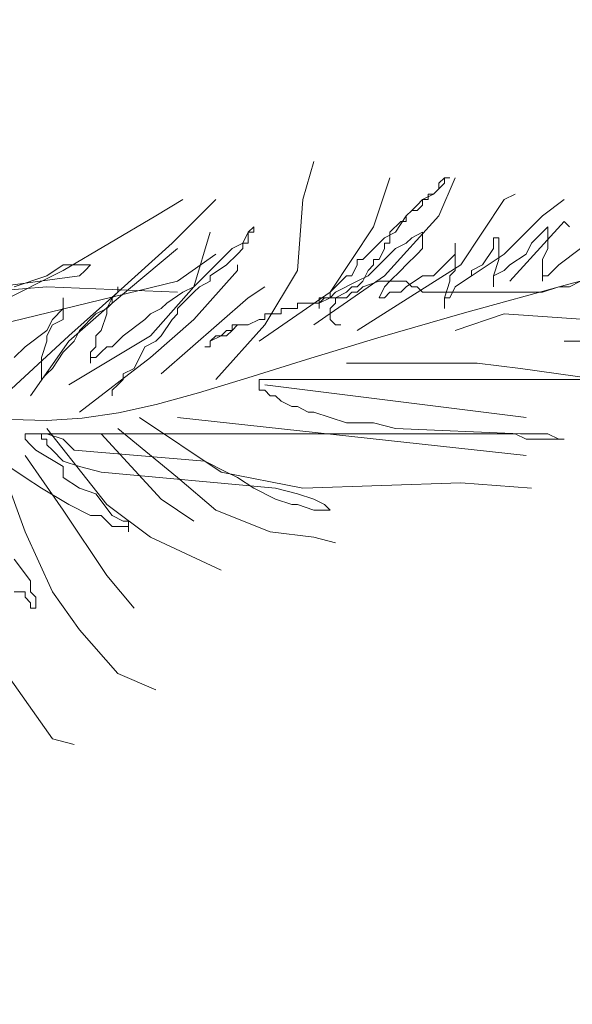
# Model space of a CAD drawing. Units: millimetres. Extents: x 595116 to 630915, y 909473 to 920225.
# Tile 59 of 134: x 629606.022 to 629608.928, y 919290.711 to 919295.882. Entities that reach past the tile are written whole.
import ezdxf

# ---------------------------------------------------------------- set-up
doc = ezdxf.new("R2010")
doc.units = ezdxf.units.MM
doc.layers.add('Dimension', color=3, linetype='Continuous', lineweight=18)
doc.layers.add('L-PLNT', color=85, linetype='Continuous', lineweight=13)
doc.styles.get("Standard").update_dxf_attribs({"font": 'arial.ttf'})
doc.dimstyles.new('ISO-25', dxfattribs={"dimtxt": 9, "dimasz": 6, "dimexe": 1.25, "dimexo": 0.625, "dimtad": 1, "dimlunit": 4, "dimtxsty": 'Standard', "dimcen": 2.5, "dimadec": 0, "dimazin": 0, "dimtfac": 1, "dimtmove": 0, "dimatfit": 3, "dimfxl": 1, "dimarcsym": 0})

# ---------------------------------------------------------------- blocks, each defined once
blk = doc.blocks.new('A$C4FB75ABC')
for p, q in [((4.2249, 2.058), (4.2402, 2.1114)), ((4.324, 2.0199), (4.3469, 2.0885)), ((4.4156, 2.0809), (4.4232, 2.0885)), ((4.4156, 2.0352), (4.4384, 2.0885)), ((4.4156, 2.0733), (4.4156, 2.0809)), ((4.4232, 2.0809), (4.4156, 2.0733)), ((4.4232, 2.0885), (4.4308, 2.0885)), ((4.4308, 2.0885), (4.4232, 2.0885)), ((4.4232, 2.0885), (4.4232, 2.0809)), ((4.4079, 2.0657), (4.4156, 2.0733)), ((4.4156, 2.0733), (4.4079, 2.0657)), ((4.019, 2.0352), (4.0571, 2.058)), ((4.0419, 1.9971), (4.1029, 2.058)), ((4.2173, 1.9589), (4.2249, 2.058)), ((4.3927, 2.058), (4.3851, 2.0504)), ((4.4079, 2.0657), (4.3927, 2.058)), ((4.3927, 2.0504), (4.3927, 2.058)), ((4.3927, 2.058), (4.4003, 2.058)), ((4.4003, 2.058), (4.4003, 2.0657)), ((4.4003, 2.0657), (4.4079, 2.0657)), ((4.4461, 1.9666), (4.5071, 2.058)), ((4.5071, 2.058), (4.5223, 2.0657)), ((4.5605, 2.0352), (4.591, 2.058)), ((4.3698, 2.0352), (4.3774, 2.0428)), ((4.3774, 2.0428), (4.3698, 2.0352)), ((4.3851, 2.0504), (4.3774, 2.0428)), ((4.3774, 2.0428), (4.3851, 2.0428)), ((4.3851, 2.0428), (4.3927, 2.0504)), ((3.8894, 1.9589), (4.019, 2.0352)), ((4.3393, 1.9513), (4.4156, 2.0352)), ((4.3469, 2.0123), (4.3622, 2.0275)), ((4.3698, 2.0352), (4.3546, 2.0123)), ((4.3622, 2.0275), (4.3698, 2.0275)), ((4.3698, 2.0275), (4.3698, 2.0352)), ((4.5071, 1.9818), (4.5605, 2.0352)), ((4.5147, 1.9437), (4.591, 2.0275)), ((4.591, 2.0275), (4.5986, 2.0199)), ((4.0724, 1.9361), (4.0953, 2.0123)), ((4.1486, 2.0123), (4.141, 1.9971)), ((4.1563, 2.0199), (4.1486, 2.0123)), ((4.1486, 1.9971), (4.1486, 2.0123)), ((4.1486, 2.0123), (4.1563, 2.0123)), ((4.1563, 2.0123), (4.1563, 2.0199)), ((4.263, 1.9285), (4.324, 2.0199)), ((4.3546, 2.0123), (4.3393, 2.0047)), ((4.3469, 1.9971), (4.3469, 2.0123)), ((4.3774, 2.0047), (4.3927, 2.0123)), ((4.3927, 2.0123), (4.3927, 1.9894)), ((4.5528, 2.0047), (4.5605, 2.0123)), ((4.5605, 2.0123), (4.5681, 2.0199)), ((4.5681, 2.0199), (4.5681, 1.9894)), ((4.3393, 2.0047), (4.3317, 1.9971)), ((4.3698, 1.9971), (4.3774, 2.0047)), ((4.4918, 1.9894), (4.4918, 2.0047)), ((4.4918, 2.0047), (4.4995, 2.0047)), ((4.4995, 2.0047), (4.4995, 1.9742)), ((4.5452, 1.9971), (4.5528, 2.0047)), ((3.958, 1.9132), (4.0495, 1.9894)), ((3.9656, 1.9285), (4.0419, 1.9971)), ((4.1258, 1.9894), (4.1181, 1.9818)), ((4.141, 1.9971), (4.1258, 1.9894)), ((4.1334, 1.9818), (4.141, 1.9894)), ((4.141, 1.9894), (4.141, 1.9971)), ((4.141, 1.9971), (4.1486, 1.9971)), ((4.3317, 1.9971), (4.3164, 1.9818)), ((4.3317, 1.9742), (4.3393, 1.9894)), ((4.3393, 1.9894), (4.3393, 1.9971)), ((4.3393, 1.9971), (4.3469, 1.9971)), ((4.3469, 1.9818), (4.3546, 1.9894)), ((4.3546, 1.9894), (4.3698, 1.9971)), ((4.3927, 1.9894), (4.3851, 1.9818)), ((4.4384, 1.9818), (4.4384, 1.9971)), ((4.4384, 1.9971), (4.4384, 1.9589)), ((4.4766, 1.9666), (4.4918, 1.9894)), ((4.5376, 1.9818), (4.5452, 1.9971)), ((4.5681, 1.9894), (4.5605, 1.9742)), ((4.5833, 1.9666), (4.6138, 1.9894)), ((4.7725, 1.9851), (4.5975, 1.9398)), ((4.0495, 1.9437), (4.1029, 1.9818)), ((4.1181, 1.9818), (4.1029, 1.9666)), ((4.1181, 1.9666), (4.1334, 1.9818)), ((4.3088, 1.9742), (4.3012, 1.9742)), ((4.3012, 1.9742), (4.3012, 1.9666)), ((4.3164, 1.9818), (4.3088, 1.9742)), ((4.3164, 1.9513), (4.3469, 1.9818)), ((4.324, 1.9666), (4.324, 1.9742)), ((4.324, 1.9742), (4.3317, 1.9742)), ((4.3851, 1.9818), (4.3698, 1.9666)), ((4.4156, 1.9589), (4.4308, 1.9742)), ((4.4308, 1.9742), (4.4384, 1.9818)), ((4.4384, 1.9361), (4.5071, 1.9818)), ((4.4995, 1.9742), (4.4918, 1.9513)), ((4.5147, 1.9666), (4.5376, 1.9818)), ((4.5605, 1.9742), (4.5605, 1.9437)), ((3.7521, 1.8903), (3.8894, 1.9589)), ((3.8894, 1.9666), (3.8665, 1.9513)), ((3.9275, 1.9666), (3.8894, 1.9666)), ((3.9122, 1.9513), (3.9199, 1.9589)), ((3.9199, 1.9589), (3.9275, 1.9666)), ((4.0724, 1.8903), (4.1334, 1.9589)), ((4.1029, 1.9666), (4.08, 1.9437)), ((4.0953, 1.9513), (4.1181, 1.9666)), ((4.1334, 1.9589), (4.1334, 1.9666)), ((4.1715, 1.8827), (4.2173, 1.9589)), ((4.3012, 1.9666), (4.2935, 1.9513)), ((4.3012, 1.8751), (4.4461, 1.9666)), ((4.3088, 1.9437), (4.3164, 1.9589)), ((4.3164, 1.9589), (4.324, 1.9666)), ((4.3622, 1.9589), (4.3469, 1.9437)), ((4.3698, 1.9666), (4.3622, 1.9589)), ((4.4079, 1.9513), (4.4156, 1.9589)), ((4.4384, 1.9589), (4.4308, 1.9513)), ((4.4613, 1.9589), (4.4766, 1.9666)), ((4.4613, 1.9513), (4.4613, 1.9589)), ((4.4918, 1.9513), (4.5071, 1.9589)), ((4.5071, 1.9589), (4.5147, 1.9666)), ((4.5681, 1.9513), (4.5757, 1.9589)), ((4.5757, 1.9589), (4.5833, 1.9666)), ((3.7445, 1.9285), (3.9122, 1.9513)), ((3.7978, 1.8827), (4.0495, 1.9437)), ((3.8665, 1.9513), (3.8207, 1.9361)), ((4.08, 1.9437), (4.0724, 1.9361)), ((4.08, 1.9361), (4.0953, 1.9437)), ((4.0953, 1.9437), (4.0953, 1.9513)), ((4.2402, 1.8827), (4.3393, 1.9513)), ((4.2859, 1.9513), (4.2707, 1.9361)), ((4.2707, 1.9285), (4.3012, 1.9437)), ((4.2935, 1.9513), (4.2859, 1.9513)), ((4.3012, 1.9437), (4.3164, 1.9513)), ((4.3012, 1.9361), (4.3088, 1.9437)), ((4.3317, 1.9437), (4.3088, 1.9361)), ((4.3698, 1.9437), (4.3317, 1.9437)), ((4.3469, 1.9437), (4.3393, 1.9361)), ((4.3698, 1.9361), (4.3927, 1.9513)), ((4.3774, 1.9361), (4.3698, 1.9437)), ((4.3927, 1.9513), (4.4079, 1.9513)), ((4.4308, 1.9437), (4.4232, 1.9208)), ((4.4308, 1.9513), (4.4308, 1.9437)), ((4.4384, 1.9361), (4.4613, 1.9513)), ((4.4918, 1.9513), (4.4918, 1.9361)), ((4.4918, 1.9361), (4.4918, 1.9513)), ((4.5605, 1.9513), (4.5681, 1.9513)), ((4.5605, 1.9437), (4.5605, 1.9513)), ((4.6138, 1.9437), (4.5986, 1.9361)), ((3.5843, 1.9132), (3.8665, 1.9361)), ((3.8665, 1.9361), (4.0495, 1.9285)), ((3.9656, 1.9285), (3.9656, 1.9361)), ((3.9656, 1.9361), (3.9656, 1.9285)), ((4.0114, 1.8675), (4.0724, 1.9361)), ((4.0724, 1.9361), (4.0571, 1.9285)), ((4.0724, 1.9285), (4.08, 1.9361)), ((4.1486, 1.9208), (4.1715, 1.9361)), ((4.2707, 1.9361), (4.263, 1.9285)), ((4.2859, 1.9285), (4.2935, 1.9361)), ((4.2935, 1.9361), (4.3012, 1.9361)), ((4.3088, 1.9361), (4.3012, 1.9285)), ((4.3393, 1.9361), (4.3317, 1.9208)), ((4.3622, 1.9285), (4.3698, 1.9361)), ((4.3851, 1.9361), (4.3774, 1.9361)), ((4.3927, 1.9285), (4.3851, 1.9361)), ((4.4308, 1.9208), (4.4384, 1.9361)), ((4.5975, 1.9398), (4.4513, 1.8996)), ((4.5833, 1.9361), (4.5605, 1.9285)), ((4.5986, 1.9361), (4.5833, 1.9361)), ((3.8894, 1.8903), (3.8894, 1.9208)), ((3.8894, 1.9208), (3.8894, 1.9056)), ((3.897, 1.8675), (3.9656, 1.9285)), ((3.958, 1.9208), (3.9504, 1.9056)), ((3.958, 1.9208), (3.9656, 1.9285)), ((3.9656, 1.9285), (3.958, 1.9208)), ((3.958, 1.9132), (3.958, 1.9208)), ((4.0266, 1.8141), (4.1486, 1.9208)), ((4.0571, 1.9285), (4.0343, 1.9132)), ((4.0571, 1.9132), (4.0724, 1.9285)), ((4.1639, 1.8599), (4.263, 1.9285)), ((4.2554, 1.9208), (4.2478, 1.9132)), ((4.2478, 1.9056), (4.2478, 1.9208)), ((4.2478, 1.9208), (4.263, 1.9208)), ((4.263, 1.9208), (4.2478, 1.9132)), ((4.263, 1.9208), (4.2554, 1.9208)), ((4.263, 1.9285), (4.263, 1.9208)), ((4.263, 1.9208), (4.2707, 1.9285)), ((4.2859, 1.9208), (4.263, 1.9208)), ((4.2707, 1.9208), (4.2859, 1.9285)), ((4.2707, 1.9132), (4.2707, 1.9208)), ((4.2935, 1.9285), (4.2859, 1.9208)), ((4.3012, 1.9285), (4.2935, 1.9285)), ((4.3317, 1.9208), (4.3393, 1.9208)), ((4.3393, 1.9208), (4.3469, 1.9285)), ((4.3469, 1.9285), (4.3622, 1.9285)), ((4.5605, 1.9285), (4.3927, 1.9285)), ((4.4232, 1.9208), (4.4232, 1.9056)), ((4.4232, 1.9056), (4.4232, 1.9208)), ((4.4232, 1.9208), (4.4308, 1.9208)), ((3.8894, 1.9056), (3.8741, 1.8903)), ((3.897, 1.8599), (3.958, 1.9132)), ((3.9504, 1.9056), (3.9351, 1.898)), ((3.9504, 1.9056), (3.958, 1.9132)), ((3.9504, 1.898), (3.9504, 1.9056)), ((4.0266, 1.9056), (4.0114, 1.898)), ((4.0343, 1.9132), (4.0266, 1.9056)), ((4.0495, 1.9056), (4.0571, 1.9132)), ((4.0495, 1.898), (4.0495, 1.9056)), ((4.2173, 1.9056), (4.1944, 1.9056)), ((4.1944, 1.9056), (4.1944, 1.898)), ((4.2478, 1.9132), (4.2173, 1.9132)), ((4.2173, 1.9132), (4.2173, 1.9056)), ((4.2478, 1.9132), (4.2478, 1.9056)), ((4.263, 1.9056), (4.2707, 1.9132)), ((4.263, 1.8903), (4.263, 1.9056)), ((3.8741, 1.8903), (3.8665, 1.8751)), ((3.8741, 1.8827), (3.8894, 1.8903)), ((3.9351, 1.898), (3.9122, 1.8751)), ((3.9427, 1.8751), (3.9504, 1.898)), ((4.0037, 1.8903), (3.9732, 1.8675)), ((4.0114, 1.898), (4.0037, 1.8903)), ((4.0114, 1.837), (4.0724, 1.8903)), ((4.0266, 1.8675), (4.0419, 1.8903)), ((4.0419, 1.8903), (4.0495, 1.898)), ((4.1639, 1.8903), (4.1486, 1.8827)), ((4.1715, 1.8903), (4.1639, 1.8903)), ((4.1944, 1.898), (4.1715, 1.898)), ((4.1715, 1.898), (4.1715, 1.8903)), ((4.2707, 1.8827), (4.263, 1.8903)), ((4.4513, 1.8996), (4.3302, 1.8644)), ((4.4384, 1.8751), (4.5071, 1.898)), ((4.5071, 1.898), (4.6215, 1.8903)), ((3.8665, 1.8751), (3.836, 1.8522)), ((3.8665, 1.8675), (3.8741, 1.8827)), ((3.9122, 1.8751), (3.9046, 1.8599)), ((3.9351, 1.8675), (3.9427, 1.8751)), ((4.1029, 1.8065), (4.1715, 1.8827)), ((4.1181, 1.8751), (4.1105, 1.8675)), ((4.1258, 1.8751), (4.1181, 1.8751)), ((4.1181, 1.8675), (4.1258, 1.8751)), ((4.1334, 1.8827), (4.1258, 1.8751)), ((4.1258, 1.8751), (4.1258, 1.8827)), ((4.1258, 1.8827), (4.1334, 1.8827)), ((4.1486, 1.8827), (4.1334, 1.8827)), ((4.2783, 1.8827), (4.2707, 1.8827)), ((3.7978, 1.776), (3.897, 1.8675)), ((3.8436, 1.7836), (3.897, 1.8599)), ((3.8589, 1.837), (3.8665, 1.8599)), ((3.8665, 1.8599), (3.8665, 1.8675)), ((3.9046, 1.8599), (3.8894, 1.8446)), ((3.897, 1.7989), (4.0114, 1.8675)), ((3.9351, 1.8522), (3.9351, 1.8675)), ((3.9656, 1.8599), (3.958, 1.8522)), ((3.9732, 1.8675), (3.9656, 1.8599)), ((4.0037, 1.8522), (4.019, 1.8599)), ((4.019, 1.8599), (4.0266, 1.8675)), ((4.1029, 1.8675), (4.0953, 1.8599)), ((4.0953, 1.8599), (4.1105, 1.8675)), ((4.0953, 1.8599), (4.0953, 1.8522)), ((4.0953, 1.8522), (4.0953, 1.8599)), ((4.1105, 1.8675), (4.1029, 1.8675)), ((4.1105, 1.8675), (4.1181, 1.8675)), ((4.3302, 1.8644), (4.2303, 1.8341)), ((4.6062, 1.8599), (4.591, 1.8599)), ((4.591, 1.8599), (4.652, 1.8599)), ((3.836, 1.8522), (3.8207, 1.837)), ((3.9275, 1.8446), (3.9351, 1.8522)), ((3.9504, 1.8522), (3.9427, 1.8446)), ((3.958, 1.8522), (3.9504, 1.8522)), ((3.9885, 1.8217), (4.0037, 1.8522)), ((4.0953, 1.8522), (4.0876, 1.8522)), ((4.0876, 1.8522), (4.0953, 1.8522)), ((3.8589, 1.8065), (3.8589, 1.837)), ((3.8894, 1.8446), (3.8741, 1.8217)), ((3.9122, 1.7608), (4.0114, 1.837)), ((3.9275, 1.8294), (3.9275, 1.8446)), ((3.9351, 1.837), (3.9275, 1.837)), ((3.9275, 1.837), (3.9275, 1.8294)), ((3.9427, 1.8446), (3.9351, 1.837)), ((4.2303, 1.8341), (4.1477, 1.8087)), ((3.8741, 1.8217), (3.8665, 1.8141)), ((3.9732, 1.8141), (3.9885, 1.8217)), ((4.2859, 1.8294), (4.4689, 1.8294)), ((4.4689, 1.8294), (4.53, 1.8217)), ((4.53, 1.8217), (4.6367, 1.8065)), ((3.8665, 1.8141), (3.8589, 1.8065)), ((3.9656, 1.7989), (3.9732, 1.8065)), ((3.9732, 1.8065), (3.9732, 1.8141)), ((4.1477, 1.8087), (4.0788, 1.7878)), ((4.1639, 1.7913), (4.1639, 1.8065)), ((4.1639, 1.8065), (5.0333, 1.8065)), ((3.958, 1.7913), (3.9656, 1.7989)), ((3.958, 1.7836), (3.958, 1.7913)), ((4.1715, 1.7913), (4.1639, 1.7913)), ((4.1715, 1.7989), (4.5376, 1.7531)), ((4.1792, 1.7836), (4.1715, 1.7913)), ((4.0788, 1.7878), (4.0197, 1.7715)), ((4.1868, 1.7836), (4.1792, 1.7836)), ((4.1944, 1.776), (4.1868, 1.7836)), ((4.0197, 1.7715), (3.9666, 1.7597)), ((4.2097, 1.7684), (4.1944, 1.776)), ((4.2173, 1.7684), (4.2097, 1.7684)), ((4.2325, 1.7608), (4.2173, 1.7684)), ((3.8664, 1.749), (3.8165, 1.7504)), ((3.916, 1.7521), (3.8664, 1.749)), ((3.9666, 1.7597), (3.916, 1.7521)), ((3.9961, 1.7531), (4.1105, 1.6769)), ((4.0495, 1.7531), (4.5376, 1.6998)), ((4.2402, 1.7608), (4.2325, 1.7608)), ((4.2859, 1.7455), (4.2402, 1.7608)), ((3.8665, 1.7379), (3.9504, 1.6312)), ((3.9656, 1.7379), (4.0495, 1.6693)), ((4.324, 1.7455), (4.2859, 1.7455)), ((4.3546, 1.7379), (4.324, 1.7455)), ((4.53, 1.7303), (4.3546, 1.7379)), ((3.836, 1.7227), (3.836, 1.7303)), ((3.836, 1.7303), (3.8665, 1.7303)), ((3.8436, 1.715), (3.836, 1.7227)), ((3.8589, 1.7227), (3.8589, 1.7303)), ((3.8589, 1.7303), (4.5223, 1.7303)), ((3.8665, 1.7227), (3.8589, 1.7227)), ((3.8665, 1.7303), (3.8894, 1.7227)), ((3.8665, 1.715), (3.8665, 1.7227)), ((3.8894, 1.7227), (3.9046, 1.7074)), ((3.9427, 1.7303), (4.0266, 1.6388)), ((4.5223, 1.7303), (4.5376, 1.7227)), ((4.5681, 1.7303), (4.53, 1.7303)), ((4.5376, 1.7227), (4.591, 1.7227)), ((4.5833, 1.7227), (4.5681, 1.7303)), ((4.591, 1.7227), (4.5833, 1.7227)), ((3.8512, 1.7074), (3.8436, 1.715)), ((3.8741, 1.7074), (3.8665, 1.715)), ((3.836, 1.6998), (3.8894, 1.6236)), ((3.8894, 1.6845), (3.8512, 1.7074)), ((3.8894, 1.6922), (3.8741, 1.7074)), ((3.9046, 1.7074), (4.0876, 1.6922)), ((3.8131, 1.6845), (3.836, 1.6693)), ((3.9122, 1.6845), (3.8894, 1.6922)), ((3.8894, 1.6693), (3.8894, 1.6845)), ((3.9427, 1.6769), (3.9122, 1.6845)), ((4.0876, 1.6922), (4.1181, 1.6769)), ((3.8055, 1.6769), (3.836, 1.5931)), ((3.836, 1.6693), (3.8589, 1.6541)), ((3.9122, 1.6541), (3.8894, 1.6693)), ((4.1868, 1.6541), (3.9427, 1.6769)), ((4.0495, 1.6693), (4.1029, 1.6236)), ((4.1105, 1.6769), (4.2249, 1.6541)), ((4.1181, 1.6769), (4.1334, 1.6693)), ((4.1334, 1.6693), (4.1563, 1.6541)), ((3.8589, 1.6541), (3.897, 1.6312)), ((3.9351, 1.6464), (3.9122, 1.6541)), ((4.1563, 1.6541), (4.1868, 1.6388)), ((4.2173, 1.6464), (4.1868, 1.6541)), ((4.2249, 1.6541), (4.4461, 1.6617)), ((4.4461, 1.6617), (4.5452, 1.6541)), ((3.958, 1.6159), (3.9351, 1.6464)), ((4.2402, 1.6388), (4.2173, 1.6464)), ((3.897, 1.6312), (3.9275, 1.6159)), ((3.9504, 1.6312), (4.0114, 1.5855)), ((4.0266, 1.6388), (4.0724, 1.6083)), ((4.1868, 1.6388), (4.2097, 1.6312)), ((4.2097, 1.6312), (4.2173, 1.6312)), ((4.2173, 1.6312), (4.2402, 1.6236)), ((4.2554, 1.6312), (4.2402, 1.6388)), ((4.263, 1.6236), (4.2554, 1.6312)), ((3.8894, 1.6236), (3.9504, 1.5321)), ((3.9275, 1.6159), (3.9427, 1.6159)), ((3.9427, 1.6159), (3.958, 1.6007)), ((3.9732, 1.6083), (3.958, 1.6159)), ((4.1029, 1.6236), (4.1792, 1.5931)), ((4.2402, 1.6236), (4.263, 1.6236)), ((3.958, 1.6007), (3.9809, 1.6007)), ((3.9809, 1.6083), (3.9732, 1.6083)), ((3.9809, 1.5931), (3.9809, 1.6083)), ((3.9809, 1.6007), (3.9809, 1.5931)), ((3.836, 1.5931), (3.8741, 1.5092)), ((4.0114, 1.5855), (4.1105, 1.5397)), ((4.1792, 1.5931), (4.2402, 1.5855)), ((4.2402, 1.5855), (4.2707, 1.5778)), ((3.8436, 1.5245), (3.8207, 1.555)), ((3.9504, 1.5321), (3.9885, 1.4864)), ((3.8436, 1.5092), (3.8436, 1.5245)), ((3.8207, 1.5092), (3.836, 1.5092)), ((3.836, 1.5092), (3.836, 1.5016)), ((3.8512, 1.5016), (3.8436, 1.5092)), ((3.8741, 1.5092), (3.9122, 1.4559)), ((3.836, 1.5016), (3.8436, 1.494)), ((3.8436, 1.494), (3.8436, 1.4864)), ((3.8512, 1.4864), (3.8512, 1.5016)), ((3.8436, 1.4864), (3.8512, 1.4864)), ((3.9122, 1.4559), (3.9656, 1.3949)), ((3.7826, 1.433), (3.8741, 1.3034)), ((3.9656, 1.3949), (4.019, 1.372)), ((3.8741, 1.3034), (3.9046, 1.2958))]:
    blk.add_line(p, q)
blk = doc.blocks.new('*D210')
at = {"layer": 'Defpoints', "color": 0, "transparency": 16777216}
for p in [(629586.2273, 919310.1229), (629593.9463, 919310.1229), (629586.2273, 919258.6624)]:
    blk.add_point(p, dxfattribs=at)
at = {"layer": 'Dimension', "color": 0, "lineweight": -2, "transparency": 16777216}
for p, q in [((629593.9463, 919310.1229), (629593.9463, 919449.6901)), ((629586.8523, 919310.1229), (629595.1963, 919310.1229)), ((629593.9463, 919264.6624), (629593.9463, 919304.1229)), ((629586.8523, 919258.6624), (629595.1963, 919258.6624))]:
    blk.add_line(p, q, dxfattribs=at)
at = {"layer": 'Dimension', "color": 0, "transparency": 16777216}
for points in [[(629592.9463, 919304.1229), (629594.9463, 919304.1229), (629593.9463, 919310.1229)], [(629592.9463, 919264.6624), (629594.9463, 919264.6624), (629593.9463, 919258.6624)]]:
    blk.add_solid(points, dxfattribs=at)
at = {"layer": 'Dimension', "color": 0, "transparency": 16777216, "insert": (629588.6617, 919382.9065), "char_height": 9, "attachment_point": 5, "rotation": 90}
blk.add_mtext('CANOPY 4\'-3 1/2" TYP.', dxfattribs=at)
blk = doc.blocks.new('*D216')
at = {"layer": 'Defpoints', "color": 0, "transparency": 16777216}
for p in [(629743.5408, 919411.9276), (629505.0408, 919411.8279), (629743.5408, 918832.3776)]:
    blk.add_point(p, dxfattribs=at)
at = {"layer": 'Dimension', "color": 0, "lineweight": -2, "transparency": 16777216}
for p, q in [((629743.5408, 919411.3026), (629743.5408, 918831.1276)), ((629505.0408, 919411.2029), (629505.0408, 918831.1276)), ((629511.0408, 918832.3776), (629737.5408, 918832.3776))]:
    blk.add_line(p, q, dxfattribs=at)
at = {"layer": 'Dimension', "color": 0, "transparency": 16777216}
for points in [[(629511.0408, 918833.3776), (629511.0408, 918831.3776), (629505.0408, 918832.3776)], [(629737.5408, 918833.3776), (629737.5408, 918831.3776), (629743.5408, 918832.3776)]]:
    blk.add_solid(points, dxfattribs=at)
at = {"layer": 'Dimension', "color": 0, "transparency": 16777216, "insert": (629624.2908, 918837.656), "char_height": 9, "attachment_point": 5}
blk.add_mtext('19\'-10 1/2"', dxfattribs=at)

msp = doc.modelspace()

# ---------------------------------------------------------------- block references
at = {"layer": 'L-PLNT', "xscale": 3.753413438031968, "yscale": 3.753413438031968, "zscale": 3.753413438031968}
msp.add_blockref('A$C4FB75ABC', (629591.6528, 919287.2124), dxfattribs=at)

# ---------------------------------------------------------------- dimensions: what is measured, and where the dimension line sits
at = {"layer": 'Dimension'}
dim = msp.add_linear_dim(base=(629593.9463, 919310.1229), p1=(629586.2273, 919258.6624), p2=(629586.2273, 919310.1229), angle=90, text='CANOPY <> TYP.', dimstyle='ISO-25', override={"dimdec": 1, "dimlfac": 1, "dimrnd": 0, "dimzin": 1, "dimdsep": 46, "dimlunit": 4, "dimfrac": 2}, dxfattribs=at)
dim.commit()
dim.dimension.update_dxf_attribs({"geometry": '*D210', "text_midpoint": (629588.6617, 919382.9065)})
dim = msp.add_linear_dim(base=(629743.5408, 918832.3776), p1=(629505.0408, 919411.8279), p2=(629743.5408, 919411.9276), dimstyle='ISO-25', override={"dimdec": 1, "dimlfac": 1, "dimrnd": 0, "dimzin": 1, "dimdsep": 46, "dimlunit": 4, "dimfrac": 2}, dxfattribs=at)
dim.commit()
dim.dimension.update_dxf_attribs({"geometry": '*D216', "text_midpoint": (629624.2908, 918837.656)})

doc.saveas('drawing.dxf')
